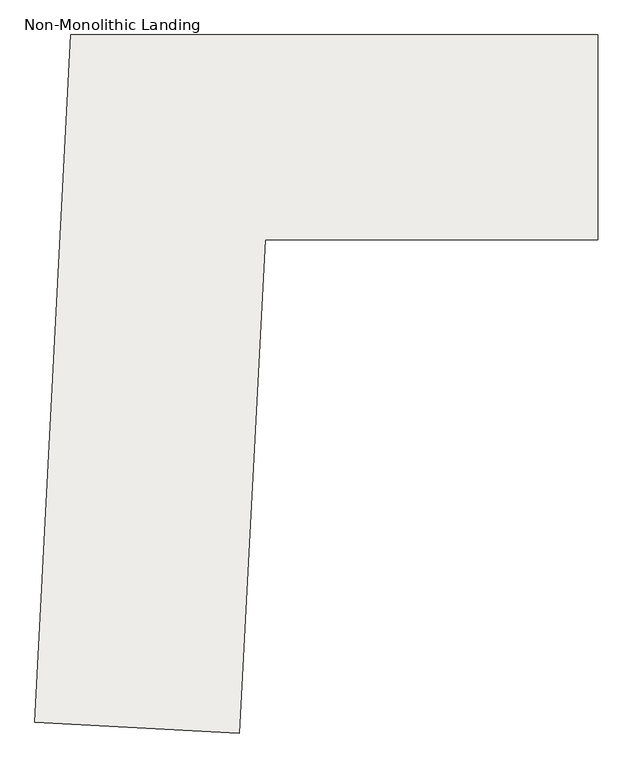
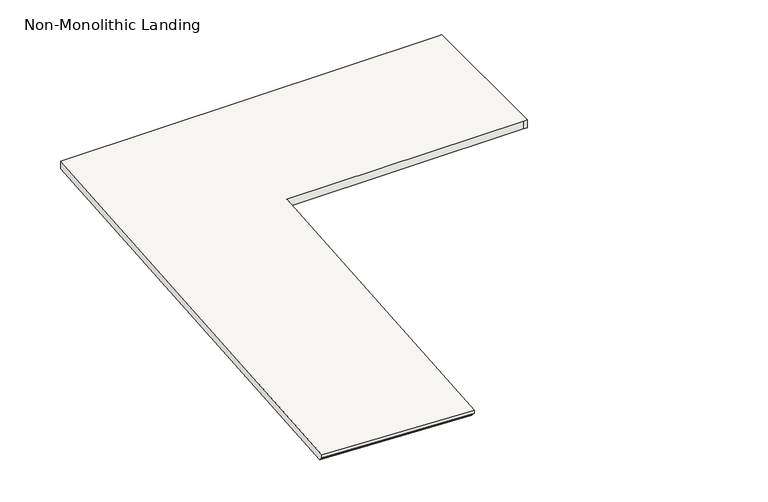
"""IFC4 building model written with IfcOpenShell, lengths in millimetres: slab geometry, Non-Monolithic Landing."""

from ifc_helpers import new_model, si_unit, origin, place, context, project, spatial, faceted_brep, source, transform, mapped, element, save


def non_monolithic_landing_6dfc5b97(model_context):
    return source(origin(), model_context, "Body", "Brep", [
        faceted_brep([(-18525.4761082, 14067.5984289, 2182.2833333), (-18525.4761082, 14067.5984289, 2201.3333333), (-19438.6229548, 14115.4544272, 2201.3333333), (-19438.6229548, 14115.4544272, 2182.2833333), (-18524.1467749, 14092.963619, 2156.8833333), (-19437.2936215, 14140.8196174, 2156.8833333), (-18409.9946473, 16271.1159704, 2201.3333333), (-16950.333929, 16271.1159704, 2201.3333333), (-16924.933929, 16271.1159704, 2201.3333333), (-16924.933929, 17185.5159704, 2201.3333333), (-16950.333929, 17185.5159704, 2201.3333333), (-19277.7278471, 17185.5159704, 2201.3333333), (-18524.1467749, 14092.963619, 2150.5333333), (-19437.2936215, 14140.8196174, 2150.5333333), (-19277.7278471, 17185.5159704, 2150.5333333), (-16950.333929, 17185.5159704, 2150.5333333), (-16924.933929, 17185.5159704, 2150.5333333), (-16924.933929, 16271.1159704, 2150.5333333), (-16950.333929, 16271.1159704, 2150.5333333), (-18409.9946473, 16271.1159704, 2150.5333333)], [[[0, 1, 2, 3]], [[4, 0, 3, 5]], [[6, 7, 8, 9, 10, 11, 2, 1]], [[12, 13, 14, 15, 16, 17, 18, 19]], [[13, 12, 4, 5]], [[6, 1, 0, 4, 12, 19]], [[7, 6, 19, 18]], [[8, 7, 18, 17]], [[9, 8, 17, 16]], [[10, 9, 16, 15]], [[11, 10, 15, 14]], [[2, 11, 14, 13, 5, 3]]]),
    ])


if __name__ == "__main__":
    model = new_model("IFC4")
    model_context = context("Model", 3, world=origin())
    ifc_project = project(units=[si_unit("LENGTHUNIT", "METRE", prefix="MILLI")], contexts=[model_context])
    site = spatial("IfcSite", under=ifc_project)
    building = spatial("IfcBuilding", under=site)
    placement = place(None, origin())
    non_monolithic_landing_shape = non_monolithic_landing_6dfc5b97(model_context)
    element("IfcSlab", 1, ObjectType="Non-Monolithic Landing", at=placement, inside=building, context=model_context, shape_type="MappedRepresentation", body=[
        mapped(non_monolithic_landing_shape, transform((0.0, 0.0, 0.0), x_axis=(1.0, 0.0, 0.0), y_axis=(0.0, 1.0, 0.0), z_axis=(0.0, 0.0, 1.0))),
    ])
    save(model, "model.ifc")
